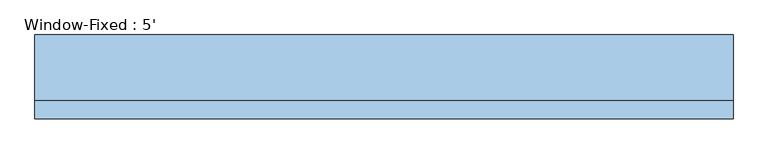
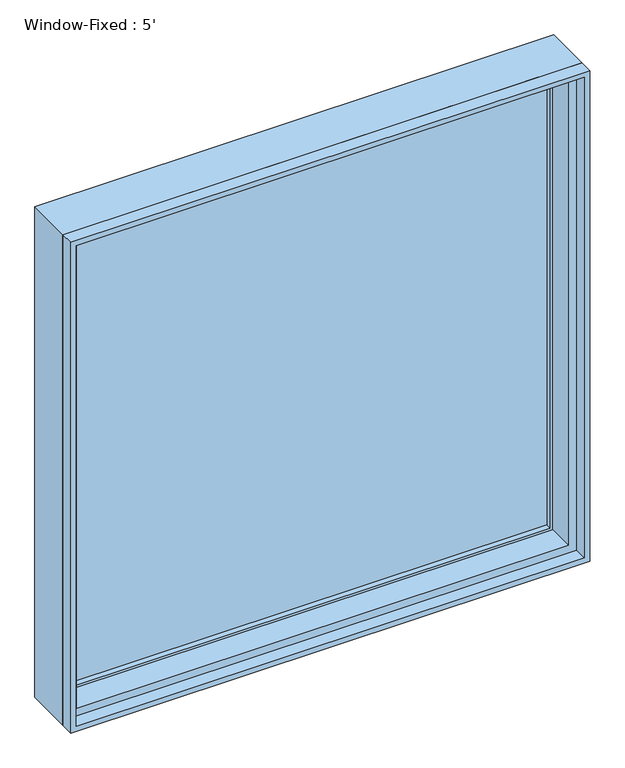
"""IFC4 building model written with IfcOpenShell, lengths in millimetres: window geometry, Window-Fixed : 5'."""

from ifc_helpers import new_model, si_unit, frame, origin, place, context, project, spatial, polyline, outline, extrude, faceted_brep, source, transform, mapped, element, save


def window_fixed_5_cc3256ea(model_context):
    return source(origin(), model_context, "Body", "SolidModel", [
        faceted_brep([(609.6, -31.75, 2133.6), (609.6, 82.55, 2133.6), (-609.6, 82.55, 2133.6), (-609.6, -31.75, 2133.6), (-609.6, 82.55, 914.4), (-609.6, -31.75, 914.4), (609.6, 82.55, 914.4), (609.6, -31.75, 914.4), (577.85, -31.75, 2101.85), (577.85, -31.75, 946.15), (-577.85, -31.75, 946.15), (-577.85, -31.75, 2101.85), (-596.9, 82.55, 2120.9), (-596.9, 82.55, 927.1), (596.9, 82.55, 927.1), (596.9, 82.55, 2120.9), (577.85, 31.75, 2101.85), (-577.85, 31.75, 2101.85), (596.9, 31.75, 2120.9), (-596.9, 31.75, 2120.9), (-577.85, 31.75, 946.15), (-596.9, 31.75, 927.1), (577.85, 31.75, 946.15), (596.9, 31.75, 927.1)], [[[0, 1, 2, 3]], [[3, 2, 4, 5]], [[5, 4, 6, 7]], [[3, 5, 7, 0], [8, 9, 10, 11]], [[7, 6, 1, 0]], [[1, 6, 4, 2], [12, 13, 14, 15]], [[16, 8, 11, 17]], [[15, 18, 19, 12]], [[17, 11, 10, 20]], [[12, 19, 21, 13]], [[20, 10, 9, 22]], [[13, 21, 23, 14]], [[22, 9, 8, 16]], [[18, 23, 21, 19], [17, 20, 22, 16]], [[14, 23, 18, 15]]]),
        extrude(outline(polyline([(2133.6, -609.6), (914.4, -609.6), (914.4, 609.6), (2133.6, 609.6), (2133.6, -609.6)]), holes=[polyline([(2120.9, 596.9), (927.1, 596.9), (927.1, -596.9), (2120.9, -596.9), (2120.9, 596.9)])]), frame((0.0, -63.5, 0.0), z_axis=(0.0, 1.0, 0.0), x_axis=(0.0, 0.0, 1.0)), (0.0, 0.0, 1.0), 31.75),
        extrude(outline(polyline([(927.1, 596.9), (2120.9, 596.9), (2120.9, -596.9), (927.1, -596.9), (927.1, 596.9)]), holes=[polyline([(952.5, -571.5), (2095.5, -571.5), (2095.5, 571.5), (952.5, 571.5), (952.5, -571.5)])]), frame((0.0, 31.75, 0.0), z_axis=(0.0, 1.0, 0.0), x_axis=(0.0, 0.0, 1.0)), (0.0, 0.0, 1.0), 44.45),
        extrude(outline(polyline([(571.5, 63.5), (571.5, 57.15), (-571.5, 57.15), (-571.5, 63.5), (571.5, 63.5)])), frame((0.0, 0.0, 952.5), z_axis=(0.0, 0.0, 1.0), x_axis=(1.0, 0.0, 0.0)), (0.0, 0.0, 1.0), 1143.0),
        extrude(outline(polyline([(-571.5, 44.45), (-571.5, 50.8), (571.5, 50.8), (571.5, 44.45), (-571.5, 44.45)])), frame((0.0, 0.0, 952.5), z_axis=(0.0, 0.0, 1.0), x_axis=(1.0, 0.0, 0.0)), (0.0, 0.0, 1.0), 1143.0),
    ])


if __name__ == "__main__":
    model = new_model("IFC4")
    model_context = context("Model", 3, world=origin())
    ifc_project = project(units=[si_unit("LENGTHUNIT", "METRE", prefix="MILLI")], contexts=[model_context])
    site = spatial("IfcSite", under=ifc_project)
    building = spatial("IfcBuilding", under=site)
    placement = place(None, origin())
    window_fixed_5_shape = window_fixed_5_cc3256ea(model_context)
    element("IfcWindow", 1, ObjectType="Window-Fixed : 5'", at=placement, inside=building, context=model_context, shape_type="MappedRepresentation", body=[
        mapped(window_fixed_5_shape, transform((0.0, 0.0, 0.0), x_axis=(1.0, 0.0, 0.0), y_axis=(0.0, 1.0, 0.0), z_axis=(0.0, 0.0, 1.0))),
    ])
    save(model, "model.ifc")

# Revit data of these elements
# Type "Window-Fixed : 5'"
#   Type Mark = "25"
#   Fire Rating = "0.5h"
#   Assembly Code = "B2020100"
#   Analytic Construction = "Double glazing - domestic"
#   Window Inset [instance default] = 0' - 0"
#   Wall Thickness [instance default] = 0' - 6"
#   Visual Light Transmittance = 0.81
#   Thermal Resistance (R) = 1.8146 (h·ft²·°F)/BTU
#   Solar Heat Gain Coefficient = 0.76
#   Rough Width = 4' - 0 1/2"
#   Rough Height = 4' - 0 1/2"
#   Interior Wall Closure [instance default] = 0' - 2 1/4"
#   Height = 4' - 0"
#   Heat Transfer Coefficient (U) = 0.5511 BTU/(h·ft²·°F)
#   Frame Extension [instance default] = 0' - 0 1/4"
#   Exterior Wall Closure [instance default] = 0' - 1 1/4"
#   Extension Jamb [instance default] = 0' - 2 1/4"
#   Default Sill Height = 3' - 0"
#   Width = 4' - 0"
#   Muntin Visibility = yes
#   Interior Trim Visibility [instance default] = yes
#   Exterior Trim Visibility [instance default] = yes
#   Extension Jamb Visibility [instance default] = yes
#   Muntin Pattern = Muntin Pattern_2x2 : Muntin Pattern_2x2
#   Interior Trim Material = Wood - Stained
#   Interior Trim = Trim-Window-Interior-Flat : Picture Frame
#   Interior Frame Material = Wood - Stained
#   Glass Panel Material = Glass
#   Exterior Trim Material = Clad - White
#   Exterior Trim = Trim-Window-Exterior-Flat : with Sill
#   Exterior Frame Material = Clad - White
#   Wall Closure = (empty or 0)
# Element 1 (IfcWindow, "Window-Fixed : 5'")
#   Wall Thickness = 0' - 5"
#   Extension Jamb = 0' - 1 1/4"
#   Materials on its faces: "Wood - Stained", "Glass", "Clad - White"
# Materials
#   "Wood - Stained": class "Wood", colour RGB 224 178 126, transparency 0, Cost = 0
#   "Glass": class "Glass", colour RGB 0 128 192, transparency 0.75, Description = "Soda Lime Glass", Cost = 0
#   "Clad - White": class "Wood", colour RGB 242 242 238, transparency 0, Cost = 0
